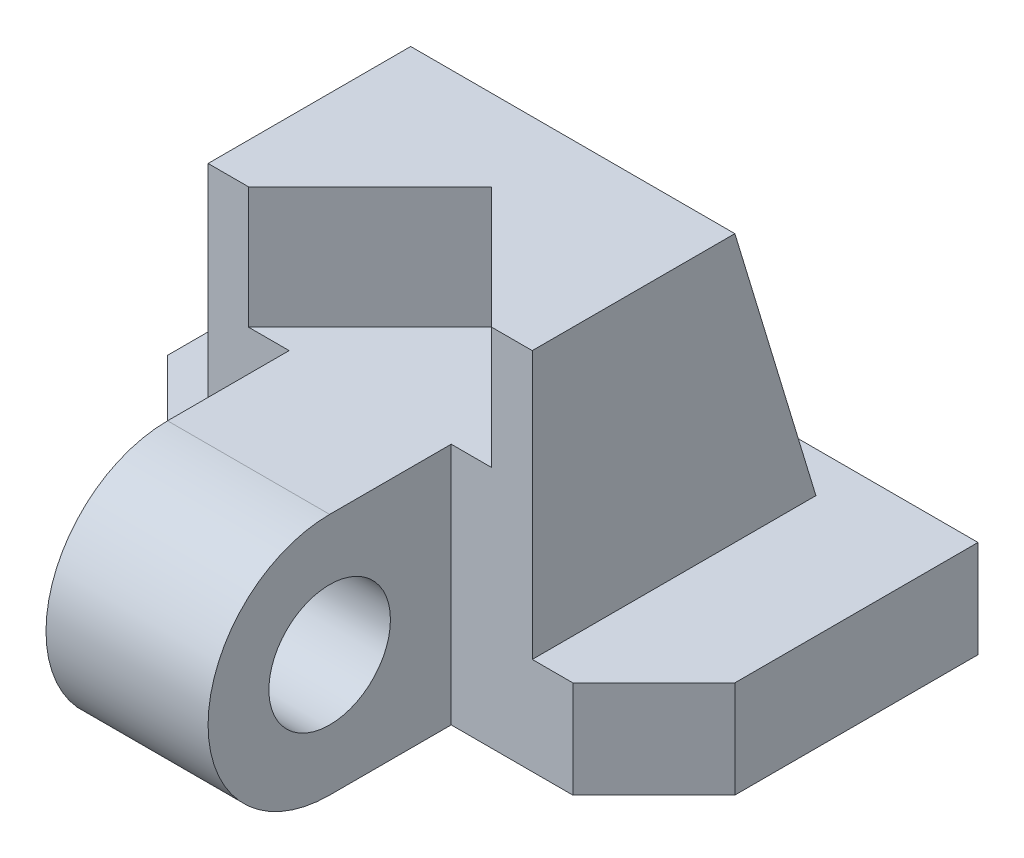
ISO-10303-21;
HEADER;
FILE_DESCRIPTION(('STEP AP214'),'2;1');
FILE_NAME('part.step','',(''),(''),'','','');
FILE_SCHEMA(('AUTOMOTIVE_DESIGN { 1 0 10303 214 1 1 1 1 }'));
ENDSEC;
DATA;
#1=APPLICATION_CONTEXT('core data for automotive mechanical design processes');
#2=APPLICATION_PROTOCOL_DEFINITION('international standard','automotive_design',2000,#1);
#3=PRODUCT_CONTEXT('',#1,'mechanical');
#4=PRODUCT('Part','Part','',(#3));
#5=PRODUCT_RELATED_PRODUCT_CATEGORY('part','',(#4));
#6=PRODUCT_DEFINITION_FORMATION('','',#4);
#7=PRODUCT_DEFINITION_CONTEXT('part definition',#1,'design');
#8=PRODUCT_DEFINITION('design','',#6,#7);
#9=PRODUCT_DEFINITION_SHAPE('','',#8);
#10=(LENGTH_UNIT() NAMED_UNIT(*) SI_UNIT(.MILLI.,.METRE.));
#11=(NAMED_UNIT(*) PLANE_ANGLE_UNIT() SI_UNIT($,.RADIAN.));
#12=(NAMED_UNIT(*) SI_UNIT($,.STERADIAN.) SOLID_ANGLE_UNIT());
#13=UNCERTAINTY_MEASURE_WITH_UNIT(LENGTH_MEASURE(1.E-05),#10,'distance_accuracy_value','');
#14=(GEOMETRIC_REPRESENTATION_CONTEXT(3) GLOBAL_UNCERTAINTY_ASSIGNED_CONTEXT((#13)) GLOBAL_UNIT_ASSIGNED_CONTEXT((#10,
#11,#12)) REPRESENTATION_CONTEXT('',''));
#15=CARTESIAN_POINT('',(0.,0.,0.));
#16=DIRECTION('',(0.,0.,1.));
#17=DIRECTION('',(1.,0.,0.));
#18=AXIS2_PLACEMENT_3D('',#15,#16,#17);
#19=CARTESIAN_POINT('',(-25.,12.,40.));
#20=DIRECTION('',(0.,0.,-1.));
#21=DIRECTION('',(-1.,0.,0.));
#22=AXIS2_PLACEMENT_3D('',#19,#20,#21);
#23=PLANE('',#22);
#24=DIRECTION('',(0.,1.,0.));
#25=VECTOR('',#24,1.);
#26=CARTESIAN_POINT('',(15.,-3.54101966249684,40.));
#27=LINE('',#26,#25);
#28=CARTESIAN_POINT('',(15.,30.,40.));
#29=VERTEX_POINT('',#28);
#30=CARTESIAN_POINT('',(15.,45.,40.));
#31=VERTEX_POINT('',#30);
#32=EDGE_CURVE('E195',#29,#31,#27,.T.);
#33=ORIENTED_EDGE('',*,*,#32,.F.);
#34=DIRECTION('',(1.,0.,0.));
#35=VECTOR('',#34,1.);
#36=CARTESIAN_POINT('',(15.,30.,40.));
#37=LINE('',#36,#35);
#38=CARTESIAN_POINT('',(10.,30.,40.));
#39=VERTEX_POINT('',#38);
#40=EDGE_CURVE('E189',#39,#29,#37,.T.);
#41=ORIENTED_EDGE('',*,*,#40,.F.);
#42=DIRECTION('',(0.,1.,0.));
#43=VECTOR('',#42,1.);
#44=CARTESIAN_POINT('',(10.,30.,40.));
#45=LINE('',#44,#43);
#46=CARTESIAN_POINT('',(10.,0.,40.));
#47=VERTEX_POINT('',#46);
#48=EDGE_CURVE('E71',#47,#39,#45,.T.);
#49=ORIENTED_EDGE('',*,*,#48,.F.);
#50=DIRECTION('',(1.,0.,0.));
#51=VECTOR('',#50,1.);
#52=CARTESIAN_POINT('',(-25.,0.,40.));
#53=LINE('',#52,#51);
#54=CARTESIAN_POINT('',(25.,0.,40.));
#55=VERTEX_POINT('',#54);
#56=EDGE_CURVE('E436',#47,#55,#53,.T.);
#57=ORIENTED_EDGE('',*,*,#56,.T.);
#58=DIRECTION('',(0.,-1.,0.));
#59=VECTOR('',#58,1.);
#60=CARTESIAN_POINT('',(25.,12.,40.));
#61=LINE('',#60,#59);
#62=CARTESIAN_POINT('',(25.,12.,40.));
#63=VERTEX_POINT('',#62);
#64=EDGE_CURVE('E450',#63,#55,#61,.T.);
#65=ORIENTED_EDGE('',*,*,#64,.F.);
#66=DIRECTION('',(1.,0.,0.));
#67=VECTOR('',#66,1.);
#68=CARTESIAN_POINT('',(-25.,12.,40.));
#69=LINE('',#68,#67);
#70=CARTESIAN_POINT('',(20.,12.,40.));
#71=VERTEX_POINT('',#70);
#72=EDGE_CURVE('E412',#71,#63,#69,.T.);
#73=ORIENTED_EDGE('',*,*,#72,.F.);
#74=DIRECTION('',(0.,-1.,0.));
#75=VECTOR('',#74,1.);
#76=CARTESIAN_POINT('',(20.,45.,40.));
#77=LINE('',#76,#75);
#78=CARTESIAN_POINT('',(20.,45.,40.));
#79=VERTEX_POINT('',#78);
#80=EDGE_CURVE('E229',#79,#71,#77,.T.);
#81=ORIENTED_EDGE('',*,*,#80,.F.);
#82=DIRECTION('',(1.,0.,0.));
#83=VECTOR('',#82,1.);
#84=CARTESIAN_POINT('',(-20.,45.,40.));
#85=LINE('',#84,#83);
#86=EDGE_CURVE('E284',#31,#79,#85,.T.);
#87=ORIENTED_EDGE('',*,*,#86,.F.);
#88=EDGE_LOOP('',(#33,#41,#49,#57,#65,#73,#81,#87));
#89=FACE_BOUND('',#88,.T.);
#90=ADVANCED_FACE('F50',(#89),#23,.F.);
#91=CARTESIAN_POINT('',(0.,12.,0.));
#92=DIRECTION('',(0.,1.,0.));
#93=DIRECTION('',(0.,0.,1.));
#94=AXIS2_PLACEMENT_3D('',#91,#92,#93);
#95=PLANE('',#94);
#96=CARTESIAN_POINT('',(-25.,12.,40.));
#97=VERTEX_POINT('',#96);
#98=CARTESIAN_POINT('',(-20.,12.,40.));
#99=VERTEX_POINT('',#98);
#100=EDGE_CURVE('E366',#97,#99,#69,.T.);
#101=ORIENTED_EDGE('',*,*,#100,.T.);
#102=DIRECTION('',(0.,0.,1.));
#103=VECTOR('',#102,1.);
#104=CARTESIAN_POINT('',(-20.,12.,40.));
#105=LINE('',#104,#103);
#106=CARTESIAN_POINT('',(-20.,12.,5.));
#107=VERTEX_POINT('',#106);
#108=EDGE_CURVE('E361',#107,#99,#105,.T.);
#109=ORIENTED_EDGE('',*,*,#108,.F.);
#110=DIRECTION('',(-1.,0.,0.));
#111=VECTOR('',#110,1.);
#112=CARTESIAN_POINT('',(-20.,12.,5.));
#113=LINE('',#112,#111);
#114=CARTESIAN_POINT('',(20.,12.,5.));
#115=VERTEX_POINT('',#114);
#116=EDGE_CURVE('E368',#115,#107,#113,.T.);
#117=ORIENTED_EDGE('',*,*,#116,.F.);
#118=DIRECTION('',(0.,0.,-1.));
#119=VECTOR('',#118,1.);
#120=CARTESIAN_POINT('',(20.,12.,5.));
#121=LINE('',#120,#119);
#122=EDGE_CURVE('E227',#71,#115,#121,.T.);
#123=ORIENTED_EDGE('',*,*,#122,.F.);
#124=ORIENTED_EDGE('',*,*,#72,.T.);
#125=DIRECTION('',(0.707106781186547,0.,-0.707106781186548));
#126=VECTOR('',#125,1.);
#127=CARTESIAN_POINT('',(25.,12.,40.));
#128=LINE('',#127,#126);
#129=CARTESIAN_POINT('',(35.,12.,30.));
#130=VERTEX_POINT('',#129);
#131=EDGE_CURVE('E430',#63,#130,#128,.T.);
#132=ORIENTED_EDGE('',*,*,#131,.T.);
#133=DIRECTION('',(0.,0.,-1.));
#134=VECTOR('',#133,1.);
#135=CARTESIAN_POINT('',(35.,12.,30.));
#136=LINE('',#135,#134);
#137=CARTESIAN_POINT('',(35.,12.,0.));
#138=VERTEX_POINT('',#137);
#139=EDGE_CURVE('E429',#130,#138,#136,.T.);
#140=ORIENTED_EDGE('',*,*,#139,.T.);
#141=DIRECTION('',(-1.,0.,0.));
#142=VECTOR('',#141,1.);
#143=CARTESIAN_POINT('',(35.,12.,0.));
#144=LINE('',#143,#142);
#145=CARTESIAN_POINT('',(-35.,12.,0.));
#146=VERTEX_POINT('',#145);
#147=EDGE_CURVE('E441',#138,#146,#144,.T.);
#148=ORIENTED_EDGE('',*,*,#147,.T.);
#149=DIRECTION('',(0.,0.,1.));
#150=VECTOR('',#149,1.);
#151=CARTESIAN_POINT('',(-35.,12.,0.));
#152=LINE('',#151,#150);
#153=CARTESIAN_POINT('',(-35.,12.,30.));
#154=VERTEX_POINT('',#153);
#155=EDGE_CURVE('E491',#146,#154,#152,.T.);
#156=ORIENTED_EDGE('',*,*,#155,.T.);
#157=DIRECTION('',(0.707106781186548,0.,0.707106781186548));
#158=VECTOR('',#157,1.);
#159=CARTESIAN_POINT('',(-35.,12.,30.));
#160=LINE('',#159,#158);
#161=EDGE_CURVE('E425',#154,#97,#160,.T.);
#162=ORIENTED_EDGE('',*,*,#161,.T.);
#163=EDGE_LOOP('',(#101,#109,#117,#123,#124,#132,#140,#148,#156,#162));
#164=FACE_BOUND('',#163,.T.);
#165=ADVANCED_FACE('F264',(#164),#95,.T.);
#166=CARTESIAN_POINT('',(0.,12.,0.));
#167=DIRECTION('',(0.,0.,1.));
#168=DIRECTION('',(1.,0.,0.));
#169=AXIS2_PLACEMENT_3D('',#166,#167,#168);
#170=PLANE('',#169);
#171=DIRECTION('',(-1.,0.,0.));
#172=VECTOR('',#171,1.);
#173=CARTESIAN_POINT('',(0.,0.,0.));
#174=LINE('',#173,#172);
#175=CARTESIAN_POINT('',(35.,0.,0.));
#176=VERTEX_POINT('',#175);
#177=CARTESIAN_POINT('',(-35.,0.,0.));
#178=VERTEX_POINT('',#177);
#179=EDGE_CURVE('E369',#176,#178,#174,.T.);
#180=ORIENTED_EDGE('',*,*,#179,.T.);
#181=DIRECTION('',(0.,-1.,0.));
#182=VECTOR('',#181,1.);
#183=CARTESIAN_POINT('',(-35.,12.,0.));
#184=LINE('',#183,#182);
#185=EDGE_CURVE('E12',#146,#178,#184,.T.);
#186=ORIENTED_EDGE('',*,*,#185,.F.);
#187=ORIENTED_EDGE('',*,*,#147,.F.);
#188=DIRECTION('',(0.,-1.,0.));
#189=VECTOR('',#188,1.);
#190=CARTESIAN_POINT('',(35.,12.,0.));
#191=LINE('',#190,#189);
#192=EDGE_CURVE('E431',#138,#176,#191,.T.);
#193=ORIENTED_EDGE('',*,*,#192,.T.);
#194=EDGE_LOOP('',(#180,#186,#187,#193));
#195=FACE_BOUND('',#194,.T.);
#196=ADVANCED_FACE('F47',(#195),#170,.F.);
#197=CARTESIAN_POINT('',(-35.,12.,0.));
#198=DIRECTION('',(1.,0.,0.));
#199=DIRECTION('',(0.,0.,-1.));
#200=AXIS2_PLACEMENT_3D('',#197,#198,#199);
#201=PLANE('',#200);
#202=DIRECTION('',(0.,0.,1.));
#203=VECTOR('',#202,1.);
#204=CARTESIAN_POINT('',(-35.,0.,0.));
#205=LINE('',#204,#203);
#206=CARTESIAN_POINT('',(-35.,0.,30.));
#207=VERTEX_POINT('',#206);
#208=EDGE_CURVE('E371',#178,#207,#205,.T.);
#209=ORIENTED_EDGE('',*,*,#208,.T.);
#210=DIRECTION('',(0.,-1.,0.));
#211=VECTOR('',#210,1.);
#212=CARTESIAN_POINT('',(-35.,12.,30.));
#213=LINE('',#212,#211);
#214=EDGE_CURVE('E60',#154,#207,#213,.T.);
#215=ORIENTED_EDGE('',*,*,#214,.F.);
#216=ORIENTED_EDGE('',*,*,#155,.F.);
#217=ORIENTED_EDGE('',*,*,#185,.T.);
#218=EDGE_LOOP('',(#209,#215,#216,#217));
#219=FACE_BOUND('',#218,.T.);
#220=ADVANCED_FACE('F396',(#219),#201,.F.);
#221=CARTESIAN_POINT('',(-35.,12.,30.));
#222=DIRECTION('',(0.707106781186547,0.,-0.707106781186547));
#223=DIRECTION('',(-0.707106781186548,0.,-0.707106781186548));
#224=AXIS2_PLACEMENT_3D('',#221,#222,#223);
#225=PLANE('',#224);
#226=DIRECTION('',(0.707106781186548,0.,0.707106781186548));
#227=VECTOR('',#226,1.);
#228=CARTESIAN_POINT('',(-35.,0.,30.));
#229=LINE('',#228,#227);
#230=CARTESIAN_POINT('',(-25.,0.,40.));
#231=VERTEX_POINT('',#230);
#232=EDGE_CURVE('E432',#207,#231,#229,.T.);
#233=ORIENTED_EDGE('',*,*,#232,.T.);
#234=DIRECTION('',(0.,-1.,0.));
#235=VECTOR('',#234,1.);
#236=CARTESIAN_POINT('',(-25.,12.,40.));
#237=LINE('',#236,#235);
#238=EDGE_CURVE('E455',#97,#231,#237,.T.);
#239=ORIENTED_EDGE('',*,*,#238,.F.);
#240=ORIENTED_EDGE('',*,*,#161,.F.);
#241=ORIENTED_EDGE('',*,*,#214,.T.);
#242=EDGE_LOOP('',(#233,#239,#240,#241));
#243=FACE_BOUND('',#242,.T.);
#244=ADVANCED_FACE('F393',(#243),#225,.F.);
#245=DIRECTION('',(0.,1.,0.));
#246=VECTOR('',#245,1.);
#247=CARTESIAN_POINT('',(-10.,30.,40.));
#248=LINE('',#247,#246);
#249=CARTESIAN_POINT('',(-10.,0.,40.));
#250=VERTEX_POINT('',#249);
#251=CARTESIAN_POINT('',(-10.,30.,40.));
#252=VERTEX_POINT('',#251);
#253=EDGE_CURVE('E196',#250,#252,#248,.T.);
#254=ORIENTED_EDGE('',*,*,#253,.T.);
#255=CARTESIAN_POINT('',(-15.,30.,40.));
#256=VERTEX_POINT('',#255);
#257=EDGE_CURVE('E65',#256,#252,#37,.T.);
#258=ORIENTED_EDGE('',*,*,#257,.F.);
#259=DIRECTION('',(0.,1.,0.));
#260=VECTOR('',#259,1.);
#261=CARTESIAN_POINT('',(-15.,-3.54101966249684,40.));
#262=LINE('',#261,#260);
#263=CARTESIAN_POINT('',(-15.,45.,40.));
#264=VERTEX_POINT('',#263);
#265=EDGE_CURVE('E173',#256,#264,#262,.T.);
#266=ORIENTED_EDGE('',*,*,#265,.T.);
#267=CARTESIAN_POINT('',(-20.,45.,40.));
#268=VERTEX_POINT('',#267);
#269=EDGE_CURVE('E51',#268,#264,#85,.T.);
#270=ORIENTED_EDGE('',*,*,#269,.F.);
#271=DIRECTION('',(0.,-1.,0.));
#272=VECTOR('',#271,1.);
#273=CARTESIAN_POINT('',(-20.,45.,40.));
#274=LINE('',#273,#272);
#275=EDGE_CURVE('E223',#268,#99,#274,.T.);
#276=ORIENTED_EDGE('',*,*,#275,.T.);
#277=ORIENTED_EDGE('',*,*,#100,.F.);
#278=ORIENTED_EDGE('',*,*,#238,.T.);
#279=EDGE_CURVE('E440',#231,#250,#53,.T.);
#280=ORIENTED_EDGE('',*,*,#279,.T.);
#281=EDGE_LOOP('',(#254,#258,#266,#270,#276,#277,#278,#280));
#282=FACE_BOUND('',#281,.T.);
#283=ADVANCED_FACE('F293',(#282),#23,.F.);
#284=CARTESIAN_POINT('',(25.,12.,40.));
#285=DIRECTION('',(-0.707106781186548,0.,-0.707106781186547));
#286=DIRECTION('',(-0.707106781186547,0.,0.707106781186548));
#287=AXIS2_PLACEMENT_3D('',#284,#285,#286);
#288=PLANE('',#287);
#289=DIRECTION('',(0.707106781186547,0.,-0.707106781186548));
#290=VECTOR('',#289,1.);
#291=CARTESIAN_POINT('',(25.,0.,40.));
#292=LINE('',#291,#290);
#293=CARTESIAN_POINT('',(35.,0.,30.));
#294=VERTEX_POINT('',#293);
#295=EDGE_CURVE('E438',#55,#294,#292,.T.);
#296=ORIENTED_EDGE('',*,*,#295,.T.);
#297=DIRECTION('',(0.,-1.,0.));
#298=VECTOR('',#297,1.);
#299=CARTESIAN_POINT('',(35.,12.,30.));
#300=LINE('',#299,#298);
#301=EDGE_CURVE('E447',#130,#294,#300,.T.);
#302=ORIENTED_EDGE('',*,*,#301,.F.);
#303=ORIENTED_EDGE('',*,*,#131,.F.);
#304=ORIENTED_EDGE('',*,*,#64,.T.);
#305=EDGE_LOOP('',(#296,#302,#303,#304));
#306=FACE_BOUND('',#305,.T.);
#307=ADVANCED_FACE('F394',(#306),#288,.F.);
#308=CARTESIAN_POINT('',(35.,12.,30.));
#309=DIRECTION('',(-1.,0.,0.));
#310=DIRECTION('',(0.,0.,1.));
#311=AXIS2_PLACEMENT_3D('',#308,#309,#310);
#312=PLANE('',#311);
#313=DIRECTION('',(0.,0.,-1.));
#314=VECTOR('',#313,1.);
#315=CARTESIAN_POINT('',(35.,0.,30.));
#316=LINE('',#315,#314);
#317=EDGE_CURVE('E442',#294,#176,#316,.T.);
#318=ORIENTED_EDGE('',*,*,#317,.T.);
#319=ORIENTED_EDGE('',*,*,#192,.F.);
#320=ORIENTED_EDGE('',*,*,#139,.F.);
#321=ORIENTED_EDGE('',*,*,#301,.T.);
#322=EDGE_LOOP('',(#318,#319,#320,#321));
#323=FACE_BOUND('',#322,.T.);
#324=ADVANCED_FACE('F489',(#323),#312,.F.);
#325=CARTESIAN_POINT('',(0.,0.,0.));
#326=DIRECTION('',(0.,1.,0.));
#327=DIRECTION('',(0.,0.,1.));
#328=AXIS2_PLACEMENT_3D('',#325,#326,#327);
#329=PLANE('',#328);
#330=ORIENTED_EDGE('',*,*,#179,.F.);
#331=ORIENTED_EDGE('',*,*,#317,.F.);
#332=ORIENTED_EDGE('',*,*,#295,.F.);
#333=ORIENTED_EDGE('',*,*,#56,.F.);
#334=DIRECTION('',(0.,0.,-1.));
#335=VECTOR('',#334,1.);
#336=CARTESIAN_POINT('',(10.,0.,40.));
#337=LINE('',#336,#335);
#338=CARTESIAN_POINT('',(10.,0.,55.));
#339=VERTEX_POINT('',#338);
#340=EDGE_CURVE('E208',#339,#47,#337,.T.);
#341=ORIENTED_EDGE('',*,*,#340,.F.);
#342=DIRECTION('',(-1.,0.,0.));
#343=VECTOR('',#342,1.);
#344=CARTESIAN_POINT('',(10.,0.,55.));
#345=LINE('',#344,#343);
#346=CARTESIAN_POINT('',(-10.,0.,55.));
#347=VERTEX_POINT('',#346);
#348=EDGE_CURVE('E211',#339,#347,#345,.T.);
#349=ORIENTED_EDGE('',*,*,#348,.T.);
#350=DIRECTION('',(0.,0.,-1.));
#351=VECTOR('',#350,1.);
#352=CARTESIAN_POINT('',(-10.,0.,40.));
#353=LINE('',#352,#351);
#354=EDGE_CURVE('E204',#347,#250,#353,.T.);
#355=ORIENTED_EDGE('',*,*,#354,.T.);
#356=ORIENTED_EDGE('',*,*,#279,.F.);
#357=ORIENTED_EDGE('',*,*,#232,.F.);
#358=ORIENTED_EDGE('',*,*,#208,.F.);
#359=EDGE_LOOP('',(#330,#331,#332,#333,#341,#349,#355,#356,#357,#358));
#360=FACE_BOUND('',#359,.T.);
#361=ADVANCED_FACE('F318',(#360),#329,.F.);
#362=CARTESIAN_POINT('',(0.,45.,0.));
#363=DIRECTION('',(0.,-1.,0.));
#364=DIRECTION('',(0.,0.,-1.));
#365=AXIS2_PLACEMENT_3D('',#362,#363,#364);
#366=PLANE('',#365);
#367=DIRECTION('',(-0.707106781186547,0.,0.707106781186547));
#368=VECTOR('',#367,1.);
#369=CARTESIAN_POINT('',(-15.,45.,40.));
#370=LINE('',#369,#368);
#371=CARTESIAN_POINT('',(0.,45.,25.));
#372=VERTEX_POINT('',#371);
#373=EDGE_CURVE('E188',#372,#264,#370,.T.);
#374=ORIENTED_EDGE('',*,*,#373,.F.);
#375=DIRECTION('',(-0.707106781186547,0.,-0.707106781186547));
#376=VECTOR('',#375,1.);
#377=CARTESIAN_POINT('',(0.,45.,25.));
#378=LINE('',#377,#376);
#379=EDGE_CURVE('E181',#31,#372,#378,.T.);
#380=ORIENTED_EDGE('',*,*,#379,.F.);
#381=ORIENTED_EDGE('',*,*,#86,.T.);
#382=DIRECTION('',(0.,0.,-1.));
#383=VECTOR('',#382,1.);
#384=CARTESIAN_POINT('',(20.,45.,40.));
#385=LINE('',#384,#383);
#386=CARTESIAN_POINT('',(20.,45.,15.));
#387=VERTEX_POINT('',#386);
#388=EDGE_CURVE('E289',#79,#387,#385,.T.);
#389=ORIENTED_EDGE('',*,*,#388,.T.);
#390=DIRECTION('',(-1.,0.,0.));
#391=VECTOR('',#390,1.);
#392=CARTESIAN_POINT('',(-20.,45.,15.));
#393=LINE('',#392,#391);
#394=CARTESIAN_POINT('',(-20.,45.,15.));
#395=VERTEX_POINT('',#394);
#396=EDGE_CURVE('E331',#387,#395,#393,.T.);
#397=ORIENTED_EDGE('',*,*,#396,.T.);
#398=DIRECTION('',(0.,0.,1.));
#399=VECTOR('',#398,1.);
#400=CARTESIAN_POINT('',(-20.,45.,40.));
#401=LINE('',#400,#399);
#402=EDGE_CURVE('E221',#395,#268,#401,.T.);
#403=ORIENTED_EDGE('',*,*,#402,.T.);
#404=ORIENTED_EDGE('',*,*,#269,.T.);
#405=EDGE_LOOP('',(#374,#380,#381,#389,#397,#403,#404));
#406=FACE_BOUND('',#405,.T.);
#407=ADVANCED_FACE('F298',(#406),#366,.F.);
#408=CARTESIAN_POINT('',(0.,-0.3784693019344,1.24894869638352));
#409=DIRECTION('',(0.,0.290007395282871,-0.957024404433474));
#410=DIRECTION('',(0.,0.957024404433474,0.290007395282871));
#411=AXIS2_PLACEMENT_3D('',#408,#409,#410);
#412=PLANE('',#411);
#413=DIRECTION('',(0.,-0.957024404433474,-0.290007395282871));
#414=VECTOR('',#413,1.);
#415=CARTESIAN_POINT('',(20.,45.,15.));
#416=LINE('',#415,#414);
#417=EDGE_CURVE('E304',#387,#115,#416,.T.);
#418=ORIENTED_EDGE('',*,*,#417,.T.);
#419=ORIENTED_EDGE('',*,*,#116,.T.);
#420=DIRECTION('',(0.,-0.957024404433474,-0.290007395282871));
#421=VECTOR('',#420,1.);
#422=CARTESIAN_POINT('',(-20.,45.,15.));
#423=LINE('',#422,#421);
#424=EDGE_CURVE('E231',#395,#107,#423,.T.);
#425=ORIENTED_EDGE('',*,*,#424,.F.);
#426=ORIENTED_EDGE('',*,*,#396,.F.);
#427=EDGE_LOOP('',(#418,#419,#425,#426));
#428=FACE_BOUND('',#427,.T.);
#429=ADVANCED_FACE('F260',(#428),#412,.T.);
#430=CARTESIAN_POINT('',(-20.,0.,0.));
#431=DIRECTION('',(-1.,0.,0.));
#432=DIRECTION('',(0.,0.,1.));
#433=AXIS2_PLACEMENT_3D('',#430,#431,#432);
#434=PLANE('',#433);
#435=ORIENTED_EDGE('',*,*,#424,.T.);
#436=ORIENTED_EDGE('',*,*,#108,.T.);
#437=ORIENTED_EDGE('',*,*,#275,.F.);
#438=ORIENTED_EDGE('',*,*,#402,.F.);
#439=EDGE_LOOP('',(#435,#436,#437,#438));
#440=FACE_BOUND('',#439,.T.);
#441=ADVANCED_FACE('F249',(#440),#434,.T.);
#442=CARTESIAN_POINT('',(20.,0.,0.));
#443=DIRECTION('',(1.,0.,0.));
#444=DIRECTION('',(0.,0.,-1.));
#445=AXIS2_PLACEMENT_3D('',#442,#443,#444);
#446=PLANE('',#445);
#447=ORIENTED_EDGE('',*,*,#80,.T.);
#448=ORIENTED_EDGE('',*,*,#122,.T.);
#449=ORIENTED_EDGE('',*,*,#417,.F.);
#450=ORIENTED_EDGE('',*,*,#388,.F.);
#451=EDGE_LOOP('',(#447,#448,#449,#450));
#452=FACE_BOUND('',#451,.T.);
#453=ADVANCED_FACE('F258',(#452),#446,.T.);
#454=CARTESIAN_POINT('',(10.,15.,55.));
#455=DIRECTION('',(-1.,0.,0.));
#456=DIRECTION('',(0.,0.,1.));
#457=AXIS2_PLACEMENT_3D('',#454,#455,#456);
#458=PLANE('',#457);
#459=ORIENTED_EDGE('',*,*,#48,.T.);
#460=DIRECTION('',(0.,0.,1.));
#461=VECTOR('',#460,1.);
#462=CARTESIAN_POINT('',(10.,30.,40.));
#463=LINE('',#462,#461);
#464=CARTESIAN_POINT('',(10.,30.,55.));
#465=VERTEX_POINT('',#464);
#466=EDGE_CURVE('E201',#39,#465,#463,.T.);
#467=ORIENTED_EDGE('',*,*,#466,.T.);
#468=CARTESIAN_POINT('',(10.,15.,55.));
#469=DIRECTION('',(1.,0.,0.));
#470=DIRECTION('',(0.,0.,1.));
#471=AXIS2_PLACEMENT_3D('',#468,#469,#470);
#472=CIRCLE('',#471,15.);
#473=EDGE_CURVE('E206',#465,#339,#472,.T.);
#474=ORIENTED_EDGE('',*,*,#473,.T.);
#475=ORIENTED_EDGE('',*,*,#340,.T.);
#476=EDGE_LOOP('',(#459,#467,#474,#475));
#477=FACE_BOUND('',#476,.T.);
#478=CARTESIAN_POINT('',(10.,15.,55.));
#479=DIRECTION('',(1.,0.,0.));
#480=DIRECTION('',(0.,0.,-1.));
#481=AXIS2_PLACEMENT_3D('',#478,#479,#480);
#482=CIRCLE('',#481,7.5);
#483=CARTESIAN_POINT('',(10.,15.,47.5));
#484=VERTEX_POINT('',#483);
#485=EDGE_CURVE('E192',#484,#484,#482,.T.);
#486=ORIENTED_EDGE('',*,*,#485,.F.);
#487=EDGE_LOOP('',(#486));
#488=FACE_BOUND('',#487,.T.);
#489=ADVANCED_FACE('F263',(#477,#488),#458,.F.);
#490=CARTESIAN_POINT('',(-10.,15.,55.));
#491=DIRECTION('',(-1.,0.,0.));
#492=DIRECTION('',(0.,0.,1.));
#493=AXIS2_PLACEMENT_3D('',#490,#491,#492);
#494=PLANE('',#493);
#495=ORIENTED_EDGE('',*,*,#253,.F.);
#496=ORIENTED_EDGE('',*,*,#354,.F.);
#497=CARTESIAN_POINT('',(-10.,15.,55.));
#498=DIRECTION('',(1.,0.,0.));
#499=DIRECTION('',(0.,0.,1.));
#500=AXIS2_PLACEMENT_3D('',#497,#498,#499);
#501=CIRCLE('',#500,15.);
#502=CARTESIAN_POINT('',(-10.,30.,55.));
#503=VERTEX_POINT('',#502);
#504=EDGE_CURVE('E214',#503,#347,#501,.T.);
#505=ORIENTED_EDGE('',*,*,#504,.F.);
#506=DIRECTION('',(0.,0.,1.));
#507=VECTOR('',#506,1.);
#508=CARTESIAN_POINT('',(-10.,30.,40.));
#509=LINE('',#508,#507);
#510=EDGE_CURVE('E213',#252,#503,#509,.T.);
#511=ORIENTED_EDGE('',*,*,#510,.F.);
#512=EDGE_LOOP('',(#495,#496,#505,#511));
#513=FACE_BOUND('',#512,.T.);
#514=CARTESIAN_POINT('',(-10.,15.,55.));
#515=DIRECTION('',(1.,0.,0.));
#516=DIRECTION('',(0.,0.,-1.));
#517=AXIS2_PLACEMENT_3D('',#514,#515,#516);
#518=CIRCLE('',#517,7.5);
#519=CARTESIAN_POINT('',(-10.,15.,47.5));
#520=VERTEX_POINT('',#519);
#521=EDGE_CURVE('E200',#520,#520,#518,.T.);
#522=ORIENTED_EDGE('',*,*,#521,.T.);
#523=EDGE_LOOP('',(#522));
#524=FACE_BOUND('',#523,.T.);
#525=ADVANCED_FACE('F467',(#513,#524),#494,.T.);
#526=CARTESIAN_POINT('',(10.,30.,40.));
#527=DIRECTION('',(0.,-1.,0.));
#528=DIRECTION('',(0.,0.,-1.));
#529=AXIS2_PLACEMENT_3D('',#526,#527,#528);
#530=PLANE('',#529);
#531=ORIENTED_EDGE('',*,*,#510,.T.);
#532=DIRECTION('',(-1.,0.,0.));
#533=VECTOR('',#532,1.);
#534=CARTESIAN_POINT('',(10.,30.,55.));
#535=LINE('',#534,#533);
#536=EDGE_CURVE('E222',#465,#503,#535,.T.);
#537=ORIENTED_EDGE('',*,*,#536,.F.);
#538=ORIENTED_EDGE('',*,*,#466,.F.);
#539=ORIENTED_EDGE('',*,*,#40,.T.);
#540=DIRECTION('',(-0.707106781186548,0.,-0.707106781186548));
#541=VECTOR('',#540,1.);
#542=CARTESIAN_POINT('',(0.,30.,25.));
#543=LINE('',#542,#541);
#544=CARTESIAN_POINT('',(0.,30.,25.));
#545=VERTEX_POINT('',#544);
#546=EDGE_CURVE('E177',#29,#545,#543,.T.);
#547=ORIENTED_EDGE('',*,*,#546,.T.);
#548=DIRECTION('',(-0.707106781186548,0.,0.707106781186548));
#549=VECTOR('',#548,1.);
#550=CARTESIAN_POINT('',(-15.,30.,40.));
#551=LINE('',#550,#549);
#552=EDGE_CURVE('E169',#545,#256,#551,.T.);
#553=ORIENTED_EDGE('',*,*,#552,.T.);
#554=ORIENTED_EDGE('',*,*,#257,.T.);
#555=EDGE_LOOP('',(#531,#537,#538,#539,#547,#553,#554));
#556=FACE_BOUND('',#555,.T.);
#557=ADVANCED_FACE('F186',(#556),#530,.F.);
#558=CARTESIAN_POINT('',(10.,15.,55.));
#559=DIRECTION('',(-1.,0.,0.));
#560=DIRECTION('',(0.,0.,1.));
#561=AXIS2_PLACEMENT_3D('',#558,#559,#560);
#562=CYLINDRICAL_SURFACE('',#561,15.);
#563=ORIENTED_EDGE('',*,*,#504,.T.);
#564=ORIENTED_EDGE('',*,*,#348,.F.);
#565=ORIENTED_EDGE('',*,*,#473,.F.);
#566=ORIENTED_EDGE('',*,*,#536,.T.);
#567=EDGE_LOOP('',(#563,#564,#565,#566));
#568=FACE_BOUND('',#567,.T.);
#569=ADVANCED_FACE('F474',(#568),#562,.T.);
#570=CARTESIAN_POINT('',(10.,15.,55.));
#571=DIRECTION('',(-1.,0.,0.));
#572=DIRECTION('',(0.,0.,1.));
#573=AXIS2_PLACEMENT_3D('',#570,#571,#572);
#574=CYLINDRICAL_SURFACE('',#573,7.5);
#575=ORIENTED_EDGE('',*,*,#485,.T.);
#576=EDGE_LOOP('',(#575));
#577=FACE_BOUND('',#576,.T.);
#578=ORIENTED_EDGE('',*,*,#521,.F.);
#579=EDGE_LOOP('',(#578));
#580=FACE_BOUND('',#579,.T.);
#581=ADVANCED_FACE('F597',(#577,#580),#574,.F.);
#582=CARTESIAN_POINT('',(0.,-3.54101966249684,25.));
#583=DIRECTION('',(0.707106781186548,0.,-0.707106781186548));
#584=DIRECTION('',(-0.707106781186548,0.,-0.707106781186548));
#585=AXIS2_PLACEMENT_3D('',#582,#583,#584);
#586=PLANE('',#585);
#587=ORIENTED_EDGE('',*,*,#32,.T.);
#588=ORIENTED_EDGE('',*,*,#379,.T.);
#589=DIRECTION('',(0.,1.,0.));
#590=VECTOR('',#589,1.);
#591=CARTESIAN_POINT('',(0.,-3.54101966249684,25.));
#592=LINE('',#591,#590);
#593=EDGE_CURVE('E171',#545,#372,#592,.T.);
#594=ORIENTED_EDGE('',*,*,#593,.F.);
#595=ORIENTED_EDGE('',*,*,#546,.F.);
#596=EDGE_LOOP('',(#587,#588,#594,#595));
#597=FACE_BOUND('',#596,.T.);
#598=ADVANCED_FACE('F178',(#597),#586,.F.);
#599=CARTESIAN_POINT('',(-15.,-3.54101966249684,40.));
#600=DIRECTION('',(-0.707106781186548,0.,-0.707106781186548));
#601=DIRECTION('',(-0.707106781186548,0.,0.707106781186548));
#602=AXIS2_PLACEMENT_3D('',#599,#600,#601);
#603=PLANE('',#602);
#604=ORIENTED_EDGE('',*,*,#593,.T.);
#605=ORIENTED_EDGE('',*,*,#373,.T.);
#606=ORIENTED_EDGE('',*,*,#265,.F.);
#607=ORIENTED_EDGE('',*,*,#552,.F.);
#608=EDGE_LOOP('',(#604,#605,#606,#607));
#609=FACE_BOUND('',#608,.T.);
#610=ADVANCED_FACE('F168',(#609),#603,.F.);
#611=CLOSED_SHELL('',(#90,#165,#196,#220,#244,#283,#307,#324,#361,#407,#429,#441,#453,#489,#525,
#557,#569,#581,#598,#610));
#612=MANIFOLD_SOLID_BREP('B2',#611);
#613=ADVANCED_BREP_SHAPE_REPRESENTATION('',(#18,#612),#14);
#614=SHAPE_DEFINITION_REPRESENTATION(#9,#613);
ENDSEC;
END-ISO-10303-21;
